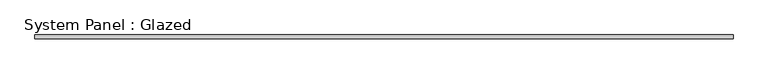
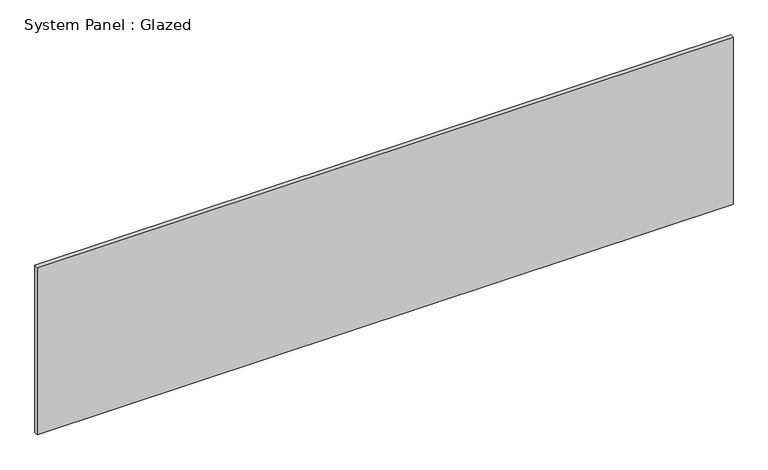
"""IFC4 building model written with IfcOpenShell, lengths in millimetres: plate geometry, System Panel : Glazed."""

from ifc_helpers import new_model, si_unit, origin, origin_with_axes, place, context, project, spatial, polyline, outline, extrude, source, transform, mapped, element, save


def system_panel_glazed_1f2a1c10(model_context):
    return source(origin(), model_context, "Body", "SweptSolid", [
        extrude(outline(polyline([(2402.2194998, 19.05), (-2402.2194998, 19.05), (-2402.2194998, 44.45), (2402.2194998, 44.45), (2402.2194998, 19.05)])), origin_with_axes(), (0.0, 0.0, 1.0), 1219.2),
    ])


if __name__ == "__main__":
    model = new_model("IFC4")
    model_context = context("Model", 3, world=origin())
    ifc_project = project(units=[si_unit("LENGTHUNIT", "METRE", prefix="MILLI")], contexts=[model_context])
    site = spatial("IfcSite", under=ifc_project)
    building = spatial("IfcBuilding", under=site)
    placement = place(None, origin())
    system_panel_glazed_shape = system_panel_glazed_1f2a1c10(model_context)
    element("IfcPlate", 1, ObjectType="System Panel : Glazed", at=placement, inside=building, context=model_context, shape_type="MappedRepresentation", body=[
        mapped(system_panel_glazed_shape, transform((0.0, 0.0, 0.0), x_axis=(1.0, 0.0, 0.0), y_axis=(0.0, 1.0, 0.0), z_axis=(0.0, 0.0, 1.0))),
    ])
    save(model, "model.ifc")

# Revit data of these elements
# Type "System Panel : Glazed"
#   Construction Type Id = "GSP4R"
#   Analytic Construction = "1/8 in Pilkington single glazing"
#   Visual Light Transmittance = 0.9
#   Solar Heat Gain Coefficient = 0.86
#   Heat Transfer Coefficient (U) = 1.18115 BTU/(h·ft²·°F)
# Element 1 (IfcPlate, "System Panel : Glazed")
#   Materials on its faces: "Glass"
# Materials
#   "Glass": class "Glass", colour RGB 0 128 192, transparency 0.75, Description = "Soda Lime Glass", Cost = 0
